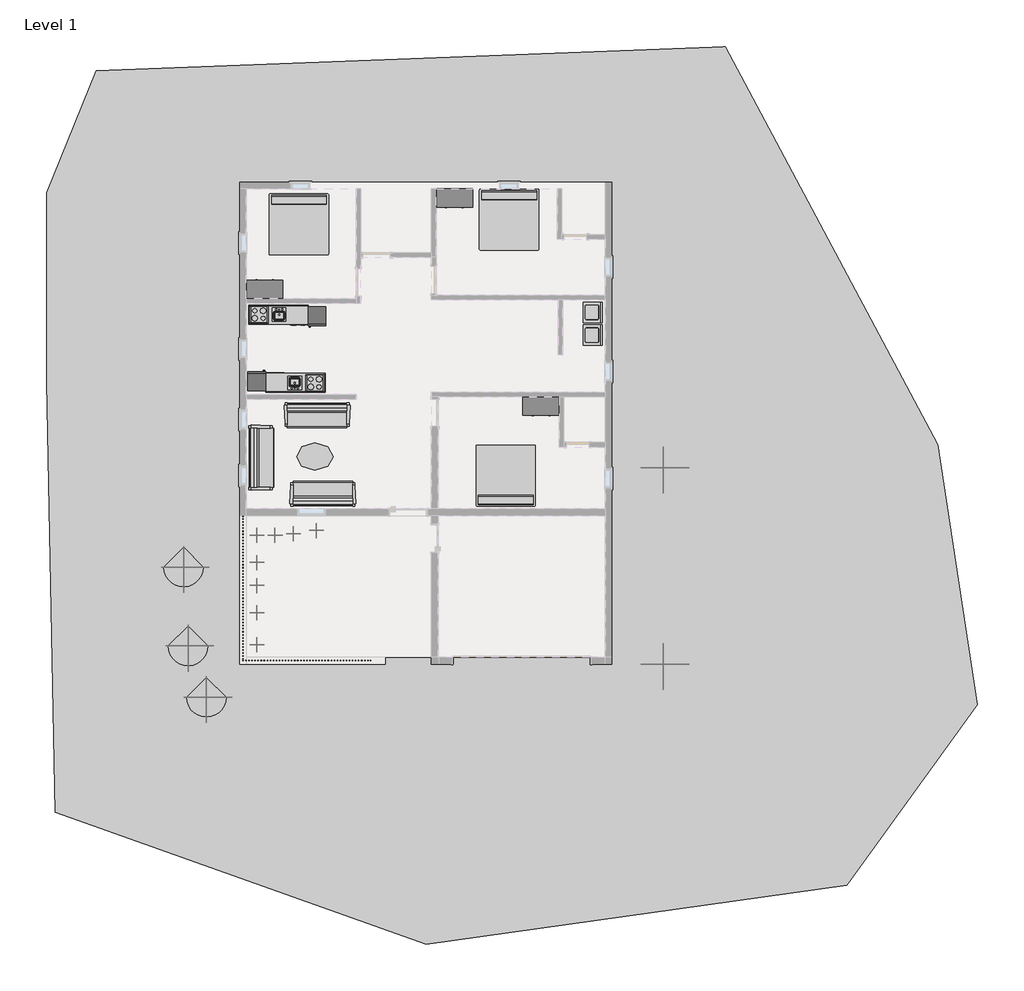
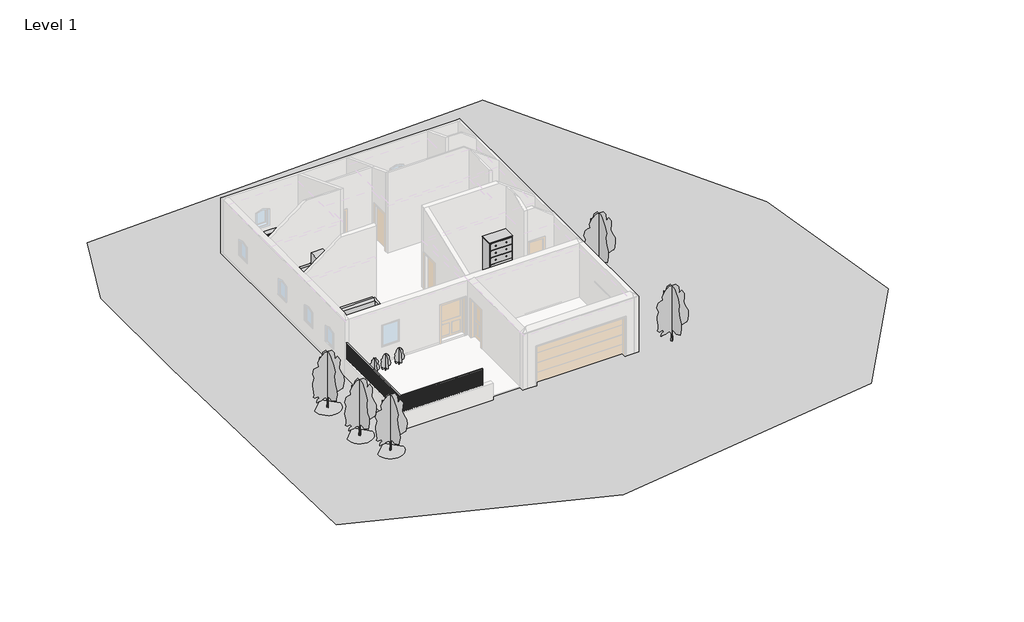
# One storey, part 3 of 3: 13 geographic elements, 12 furniture elements, 11 proxies, 2 flow terminals, 1 railing.
# Revit data of these elements (continued)
# Elements 19, 20, 21 (IfcFurniture, "Dresser : 48\" x 72\" x 24\"")
#   Phase Created = New Construction
#   Materials on its faces: "Laminate, Ivory, Matte", "Cherry", "Laminate - Ivory, Glossy"
# Elements 22, 23, 24 (IfcFurniture, "Sofa-Pensi : 84\"")
#   Phase Created = New Construction
#   Materials on its faces: "Cherry", "Linen, Beige", "Steel, Chrome Plated"
# Element 25 (IfcFurniture, "Table-Ellipse : 60\" x 48\"")
#   Phase Created = New Construction
#   Materials on its faces: "Birch"
# Elements 26, 27, 28, 29, 30 (IfcGeographicElement, "RPC Tree - Deciduous : 10' 2")
#   Phase Created = New Construction
# Elements 31, 32, 33, 34, 35, 36, 37, 38 (IfcGeographicElement, "RPC Tree - Deciduous : Red Ash - 25'")
#   Phase Created = New Construction
# Element 39 (IfcRailing, "Handrail - Rectangular")
#   built-in parameter 1008621 = 3 (stored number, unit not read)
#   Phase Created = New Construction
# Materials
#   "Steel, Chrome Plated": class "Metal", colour RGB 17 17 17, transparency 0, Description = "Chromiuim plated steel", Cost = 0
#   "Steel, Polished": class "Metal", colour RGB 57 57 57, transparency 0, Description = "Polished steel", Cost = 0
#   "Steel, Paint Finish, Ivory, Glossy": class "Metal", colour RGB 247 247 239, transparency 0, Description = "Steel, paint finish, ivory, glossy", Cost = 0
#   "Plastic, Opaque Black": class "Plastic", colour RGB 0 0 0, transparency 0.7, Description = "Plastic, generic, opaque black", Cost = 0
#   "Cabinets": colour RGB 249 249 249, transparency 0
#   "Cabinets - Handles": class "Metal", colour RGB 57 57 57, transparency 0
#   "Steel, Paint Finish, Ivory, Matte": class "Metal", colour RGB 247 247 239, transparency 0, Description = "Steel, paint finish, ivory, matte", Cost = 0
#   "Linen, White": class "Textile", colour RGB 247 247 239, transparency 0, Description = "Linen, white", Cost = 0
#   "Laminate - Ivory, Glossy": colour RGB 247 247 239, transparency 0
#   "Laminate, Ivory, Matte": class "Plastic", colour RGB 247 247 239, transparency 0, Description = "Plastic Laminate - Ivory, Matte", Cost = 0
#   "Cherry": class "Wood", colour RGB 226 177 128, transparency 0, Description = "Prunus Serotina", Cost = 0
#   "Linen, Beige": class "Textile", colour RGB 249 239 230, transparency 0, Description = "Linen, beige", Cost = 0
#   "Birch": class "Wood", colour RGB 224 178 126, transparency 0, Description = "Betula Alleghaniensis", Cost = 0
#   "GRASS": class "Generic", colour RGB 127 136 91, transparency 0, Cost = 0
#   "Counter Top": class "Wood", colour RGB 226 177 128, transparency 0
